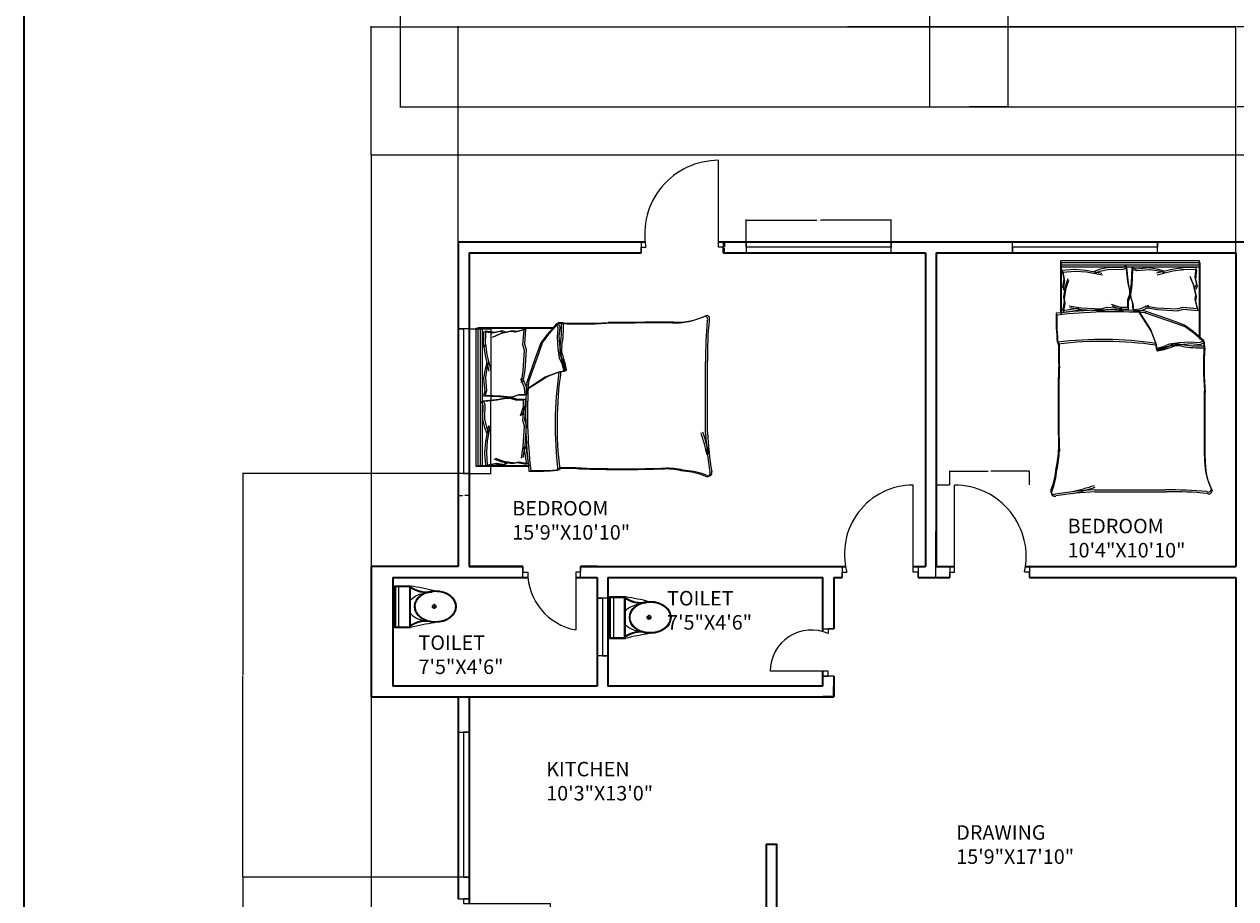
# Model space of a CAD drawing. Units: inches. Extents: x 1520 to 3401, y 1570 to 3432.
# Tile 5 of 15: x 1520 to 2022, y 2425 to 2787. Entities that reach past the tile are written whole.
import ezdxf

# ---------------------------------------------------------------- set-up
doc = ezdxf.new("R2010")
doc.units = ezdxf.units.IN
for name, color, linetype, lineweight in [('A-ANNO-DIMS', 2, 'Continuous', 18), ('A-ANNO-TTLB', 7, 'Continuous', 35), ('A-AREA-IDEN', 7, 'Continuous', 18), ('A-DOOR', 3, 'Continuous', 18), ('A-FLOR-EDGE', 7, 'Continuous', 25), ('A-FLOR-FIXT', 9, 'Continuous', 18), ('A-FURN', 8, 'Continuous', 13), ('A-GLAZ', 4, 'Continuous', 18), ('A-WALL', 7, 'Continuous', 35)]:
    doc.layers.add(name, color=color, linetype=linetype, lineweight=lineweight)
doc.styles.get("Standard").update_dxf_attribs({"font": 'arial.ttf'})
doc.dimstyles.get("Standard").update_dxf_attribs({"dimtxt": 0.18, "dimasz": 0.18, "dimexe": 0.18, "dimexo": 0.0625, "dimgap": 0.09, "dimtad": 0, "dimtih": 1, "dimtoh": 1, "dimdec": 4, "dimzin": 0, "dimdsep": 46, "dimtxsty": 'Standard', "dimcen": 0.09, "dimadec": 0, "dimazin": 0, "dimtfac": 1, "dimtdec": 4, "dimtofl": 0, "dimtmove": 0, "dimatfit": 3, "dimfxl": 1, "dimtolj": 1, "dimtzin": 0, "dimarcsym": 0})

# ---------------------------------------------------------------- blocks, each defined once
blk = doc.blocks.new('A$C31115884')
for p, q in [((283, 498), (223, 498)), ((258, 466), (258, 523)), ((0, 200), (0, 0)), ((520, 200), (0, 200)), ((10, 190), (10, 10)), ((510, 190), (10, 190)), ((510, 10), (510, 190)), ((520, 0), (520, 200)), ((510, 54), (0, 54)), ((10, 10), (510, 10)), ((0, 0), (520, 0))]:
    blk.add_line(p, q)
blk.add_circle((256, 496), 23.6)
for centre, radius, start, end in [((2778, -205), 2807, 165.4549, 171.7133), ((-295, 403), 365, 324.2091, 9.3499), ((-295, 403), 375, 324.2091, 9.3499), ((806, 403), 365, 170.6501, 215.7909), ((3237, 905), 2807, 188.2867, 194.5451), ((384, 406), 293, 190.2774, 224.1564), ((139, 406), 293, 315.8436, 2.6563), ((806, 403), 375, 179.2036, 215.7909)]:
    blk.add_arc(centre, radius, start, end)
blk.add_ellipse((256, 510), major_axis=(0, -261), ratio=0.772727)
blk.add_open_spline([(256, 259), (263, 259), (270, 260), (288, 262), (299, 265), (320, 273), (330, 278), (350, 291), (360, 299), (378, 316), (386, 326), (402, 347), (409, 358), (421, 383), (427, 395), (436, 422), (440, 436), (445, 465), (447, 480), (448, 509), (448, 524), (445, 553), (443, 568), (436, 596), (432, 610), (422, 636), (416, 649), (402, 672), (395, 683), (379, 703), (370, 712), (351, 728), (341, 735), (321, 746), (310, 751), (289, 757), (278, 759), (256, 761), (245, 761), (223, 757), (212, 754), (191, 746), (181, 741), (161, 728), (151, 720), (133, 703), (125, 693), (110, 672), (103, 660), (90, 636), (85, 623), (76, 596), (72, 582), (67, 553), (66, 538), (64, 509), (65, 494), (68, 465), (70, 450), (77, 422), (81, 408), (91, 382), (97, 370), (111, 346), (118, 335), (135, 316), (144, 307), (162, 291), (172, 284), (193, 273), (203, 269), (225, 262), (236, 260), (250, 259), (253, 259), (256, 259)], degree=3, knots=[0, 0, 0, 0, 0.110105, 0.110105, 0.285049, 0.285049, 0.459994, 0.459994, 0.634938, 0.634938, 0.809882, 0.809882, 0.984827, 0.984827, 1.159771, 1.159771, 1.334715, 1.334715, 1.50966, 1.50966, 1.684604, 1.684604, 1.859549, 1.859549, 2.034493, 2.034493, 2.209437, 2.209437, 2.384382, 2.384382, 2.559326, 2.559326, 2.73427, 2.73427, 2.909215, 2.909215, 3.084159, 3.084159, 3.259103, 3.259103, 3.434048, 3.434048, 3.608992, 3.608992, 3.783936, 3.783936, 3.958881, 3.958881, 4.133825, 4.133825, 4.30877, 4.30877, 4.483714, 4.483714, 4.658658, 4.658658, 4.833603, 4.833603, 5.008547, 5.008547, 5.183491, 5.183491, 5.358436, 5.358436, 5.53338, 5.53338, 5.708324, 5.708324, 5.883269, 5.883269, 6.058213, 6.058213, 6.233158, 6.233158, 6.283185, 6.283185, 6.283185, 6.283185])
blk = doc.blocks.new('DOOR-SWING-24-01')
for p, q in [((21.75, 19.61), (26.25, 19.61)), ((26.25, 19.61), (24, 19.61)), ((24, 19.61), (24, 17.61)), ((24, 2), (0, 2)), ((24, 0), (24, 2)), ((26.25, 0), (21.75, 0)), ((21.75, 0), (24, 0))]:
    blk.add_line(p, q)
blk.add_arc((17.08, 2), 17.08, 66.0978, 180)
blk = doc.blocks.new('DOOR-SWING-24-02')
for p, q in [((0, 21.75), (0, 26.25)), ((0, 26.25), (0, 24)), ((23.89, 21.75), (23.89, 26.25)), ((23.89, 26.25), (23.89, 24)), ((0, 24), (2, 24)), ((23.89, 24), (21.89, 24)), ((21.89, 24), (21.89, 0))]:
    blk.add_line(p, q)
blk.add_arc((26.42, 24), 24.42, 180, 259.3013)
blk = doc.blocks.new('DOOR-SWING-36-03')
for p, q in [((29.45, 2.25), (29.45, 38.25)), ((0, 4.5), (0, 0)), ((0, 0), (0, 2.25)), ((0, 2.25), (2, 2.25)), ((31.45, 2.25), (29.45, 2.25)), ((31.45, 4.5), (31.45, 0)), ((31.45, 0), (31.45, 2.25))]:
    blk.add_line(p, q)
blk.add_arc((29.45, 9.79), 28.46, 90, 195.3561)
blk = doc.blocks.new('DOOR-SWING-36-04')
for p, q in [((2, 2.25), (2, 38.25)), ((0, 4.5), (0, 0)), ((0, 0), (0, 2.25)), ((0, 2.25), (2, 2.25)), ((32.99, 2.25), (30.99, 2.25)), ((32.99, 4.5), (32.99, 0)), ((32.99, 0), (32.99, 2.25))]:
    blk.add_line(p, q)
blk.add_arc((2, 8.58), 29.67, 347.6919, 90)
blk = doc.blocks.new('DOOR-SWING-36-22')
for p, q in [((32.08, 2.25), (32.08, 38.25)), ((0, 4.5), (0, 0)), ((0, 0), (0, 2.25)), ((0, 2.25), (2, 2.25)), ((34.08, 2.25), (32.08, 2.25)), ((34.08, 4.5), (34.08, 0)), ((34.08, 0), (34.08, 2.25))]:
    blk.add_line(p, q)
blk.add_arc((32.08, 7.69), 30.56, 90, 190.2449)
blk = doc.blocks.new('DOOR-SWING-36-24')
for p, q in [((0, 30.42), (4.5, 30.42)), ((4.5, 30.42), (2.25, 30.42)), ((2.25, 30.42), (2.25, 28.42)), ((2.25, 28.42), (38.25, 28.42)), ((4.5, 0), (0, 0)), ((0, 0), (2.25, 0)), ((2.25, 0), (2.25, 2))]:
    blk.add_line(p, q)
blk.add_arc((10.55, 28.42), 27.7, 252.5577, 0)
blk = doc.blocks.new('WIN-PLAN-24-01')
for p, q in [((0, 4.5), (0, 0)), ((0, 0), (0, 2.25)), ((0, 2.25), (24, 2.25)), ((24, 2.25), (24, 4.5)), ((24, 4.5), (24, 0))]:
    blk.add_line(p, q)
blk = doc.blocks.new('WIN-PLAN-60-02')
for p, q in [((4.5, 60), (0, 60)), ((0, 60), (2.25, 60)), ((2.25, 60), (2.25, 0)), ((4.5, 0), (0, 0)), ((2.25, 0), (4.5, 0))]:
    blk.add_line(p, q)
blk = doc.blocks.new('WIN-PLAN-60-03')
for p, q in [((0, 2.25), (0, 4.5)), ((0, 4.5), (0, 0)), ((60, 2.25), (0, 2.25)), ((60, 0), (60, 4.5)), ((60, 4.5), (60, 2.25))]:
    blk.add_line(p, q)
blk = doc.blocks.new('BED-DOUBLE')
for p, q in [((4.17, 75.93), (4.17, 97.64)), ((4.17, 97.64), (61.46, 97.64)), ((4.17, 95.8), (61.46, 95.8)), ((4.44, 75.16), (4.44, 96.87)), ((4.44, 96.87), (61.73, 96.87)), ((29.42, 94.7), (31.15, 95.4)), ((31.15, 95.4), (31.84, 88.98)), ((61.46, 97.64), (61.46, 65.74)), ((61.73, 96.87), (61.73, 64.97)), ((4.44, 95.03), (61.73, 95.03)), ((4.67, 93.64), (9.81, 94.03)), ((4.67, 93.66), (5.36, 89.85)), ((4.94, 92.9), (5.64, 89.08)), ((4.95, 92.87), (10.08, 93.27)), ((9.81, 94.03), (9.93, 94.01)), ((9.93, 94.01), (14.52, 93.66)), ((10.08, 93.27), (10.21, 93.24)), ((10.21, 93.24), (14.79, 92.9)), ((14.52, 93.66), (21.1, 92.45)), ((14.79, 92.9), (21.38, 91.68)), ((17.81, 93.14), (20.24, 94.01)), ((18.08, 92.38), (20.51, 93.24)), ((20.24, 94.01), (23.7, 94.88)), ((20.51, 93.24), (23.98, 94.11)), ((23.7, 94.88), (24.09, 94.88)), ((23.98, 94.11), (24.36, 94.11)), ((24.09, 94.88), (29.42, 94.7)), ((24.36, 94.11), (29.69, 93.94)), ((29.69, 93.94), (31.42, 94.63)), ((31.42, 94.63), (32.12, 88.22)), ((33.54, 94.65), (33.25, 88.21)), ((33.81, 93.88), (33.52, 87.44)), ((35.31, 94.07), (33.54, 94.65)), ((35.59, 93.3), (33.81, 93.88)), ((40.62, 94.57), (35.31, 94.07)), ((40.9, 93.81), (35.59, 93.3)), ((41.01, 94.6), (40.62, 94.57)), ((41.28, 93.83), (40.9, 93.81)), ((44.52, 93.95), (41.01, 94.6)), ((44.79, 93.18), (41.28, 93.83)), ((50.25, 93.96), (43.75, 92.34)), ((50.52, 93.19), (44.03, 91.57)), ((47, 93.23), (44.52, 93.95)), ((47.27, 92.47), (44.79, 93.18)), ((54.8, 94.59), (50.25, 93.96)), ((55.08, 93.82), (50.52, 93.19)), ((60.08, 94.57), (53.6, 94.69)), ((53.6, 94.69), (54.8, 94.59)), ((60.35, 93.81), (53.87, 93.92)), ((53.87, 93.92), (55.08, 93.82)), ((59.12, 87.74), (57.7, 90.95)), ((60.08, 94.57), (59.62, 90.72)), ((59.62, 90.72), (60.34, 87.64)), ((60.35, 93.81), (59.9, 89.96)), ((5.36, 89.85), (4.84, 86.73)), ((4.84, 86.73), (5.54, 85.52)), ((5.64, 89.08), (5.12, 85.96)), ((5.12, 85.96), (5.81, 84.75)), ((5.36, 82.57), (6.06, 86.9)), ((5.64, 81.8), (6.33, 86.14)), ((6.06, 86.9), (7.27, 90.2)), ((6.33, 86.14), (7.54, 89.43)), ((31.84, 88.98), (32.54, 85.17)), ((32.12, 88.22), (32.81, 84.4)), ((33.25, 88.21), (32.79, 84.36)), ((33.52, 87.44), (33.07, 83.59)), ((59.39, 86.97), (57.97, 90.18)), ((60.08, 83.46), (59.12, 87.74)), ((60.35, 82.69), (59.39, 86.97)), ((60.34, 87.64), (59.72, 86.39)), ((59.9, 89.96), (60.61, 86.88)), ((60.61, 86.88), (59.99, 85.62)), ((5.02, 76.85), (5.71, 80.66)), ((5.71, 80.66), (5.36, 82.57)), ((5.98, 79.9), (5.64, 81.8)), ((32.54, 83.61), (31.84, 81.36)), ((31.84, 81.36), (31.84, 78.14)), ((32.81, 82.84), (32.12, 80.59)), ((32.12, 80.59), (32.12, 77.37)), ((32.54, 85.17), (32.54, 83.61)), ((32.79, 84.36), (32.89, 82.8)), ((32.81, 84.4), (32.81, 82.84)), ((32.89, 82.8), (33.72, 80.59)), ((33.07, 83.59), (33.17, 82.03)), ((33.17, 82.03), (34, 79.83)), ((33.72, 80.59), (33.93, 77.39)), ((59.85, 81.53), (60.08, 83.46)), ((60.78, 77.77), (59.85, 81.53)), ((60.12, 80.77), (60.35, 82.69)), ((61.05, 77), (60.12, 80.77)), ((11.13, 77.72), (5.02, 76.85)), ((5.29, 76.08), (5.98, 79.9)), ((11.4, 76.95), (5.29, 76.08)), ((7.65, 78.9), (12.48, 78.1)), ((7.92, 78.14), (12.76, 77.34)), ((12.48, 78.1), (11.13, 77.72)), ((12.76, 77.34), (11.4, 76.95)), ((12.48, 78.1), (20.89, 77.59)), ((12.76, 77.34), (21.16, 76.82)), ((20.89, 77.59), (23.24, 78.25)), ((21.16, 76.82), (23.51, 77.49)), ((23.24, 78.25), (29.39, 77.77)), ((23.51, 77.49), (29.67, 77)), ((28.9, 78.14), (25.13, 79.45)), ((29.17, 77.37), (25.4, 78.68)), ((31.84, 78.14), (28.9, 78.14)), ((32.12, 77.37), (29.17, 77.37)), ((33.93, 77.39), (36.87, 77.57)), ((34, 79.83), (34.2, 76.62)), ((34.2, 76.62), (37.14, 76.8)), ((36.28, 76.8), (41.3, 69.01)), ((36.55, 76.03), (41.57, 68.25)), ((36.87, 77.57), (40.55, 79.11)), ((37.14, 76.8), (40.82, 78.34)), ((48.73, 73.28), (38.73, 76.8)), ((49, 72.52), (39, 76.03)), ((39.04, 78.9), (43.87, 78.1)), ((39.31, 78.14), (44.15, 77.34)), ((43.87, 78.1), (52.28, 77.59)), ((44.15, 77.34), (52.55, 76.82)), ((52.28, 77.59), (54.63, 78.25)), ((52.55, 76.82), (54.9, 77.49)), ((54.63, 78.25), (60.78, 77.77)), ((54.9, 77.49), (61.05, 77)), ((55.41, 70.87), (48.73, 73.28)), ((55.69, 70.1), (49, 72.52)), ((58.94, 68.27), (55.41, 70.87)), ((41.3, 69.01), (43.34, 63.63)), ((41.57, 68.25), (43.62, 62.87)), ((59.21, 67.51), (55.69, 70.1)), ((63.38, 64.38), (58.94, 68.27)), ((63.66, 63.61), (59.21, 67.51)), ((43.34, 63.63), (43.71, 61.22)), ((43.62, 62.87), (43.99, 60.45)), ((43.71, 61.22), (46.68, 61.96)), ((43.99, 60.45), (46.96, 61.2)), ((46.68, 61.96), (49.1, 63.08)), ((46.96, 61.2), (49.37, 62.31)), ((49.1, 63.08), (53.18, 63.63)), ((49.37, 62.31), (53.46, 62.87)), ((53.18, 63.63), (57.82, 64)), ((53.46, 62.87), (58.1, 63.24)), ((57.82, 64), (61.54, 63.63)), ((58.1, 63.24), (61.81, 62.87)), ((61.54, 63.63), (63.38, 64.38)), ((61.81, 62.87), (63.66, 63.61)), ((63.48, 62.28), (63.38, 64.38, 4.64)), ((63.75, 61.52), (63.66, 63.61, 4.64)), ((18.06, 2.64), (47.57, 2.64)), ((18.33, 1.87), (47.84, 1.87))]:
    blk.add_line(p, q)
for centre, radius, start, end in [((102.1, 73.55), 99.87, 178.7218, 185.604), ((25.61, -120.62), 197.77, 86.0865, 96.7821), ((25.88, -121.38), 197.77, 86.0865, 96.7821), ((102.37, 72.78), 99.87, 178.7218, 185.604), ((21.29, -89.76), 154.68, 81.7845, 96.9006), ((21.56, -90.53), 154.68, 81.7845, 96.9006), ((-200.58, 60.27), 203.94, 358.4762, 1.0082), ((-200.3, 59.5), 203.94, 358.4762, 1.0082), ((43.92, 61.15), 0.221, 160.2464, 271.1377), ((37.35, 95.86), 35.55, 280.6617, 289.8806), ((44.2, 60.38), 0.221, 160.2464, 271.1377), ((37.62, 95.1), 35.55, 280.6617, 289.8806), ((52.44, 55.6), 7.46, 78.6608, 113.7384), ((52.72, 54.83), 7.46, 78.6608, 113.7384), ((61.53, 105.62), 43.38, 259.8763, 272.5657), ((61.81, 104.85), 43.38, 259.8763, 272.5657), ((218.51, 54.1), 155.25, 176.9791, 183.8365), ((218.79, 53.34), 155.25, 176.9791, 183.8365), ((581.23, 36.96), 578.22, 178.22771, 181.71854), ((581.51, 36.19), 578.22, 178.22771, 181.71854), ((-5405.34, 16.33), 5469.02, 0.00217, 0.28689), ((-5405.07, 15.56), 5469.02, 0.00217, 0.28689), ((-32.25, 20.29), 35.53, 346.0648, 358.9113), ((-31.97, 19.53), 35.53, 346.0648, 358.9113), ((91.3, 15.32), 27.65, 177.4714, 206.4681), ((91.58, 14.55), 27.65, 177.4714, 206.4681), ((-25.97, 13.39), 28.25, 337.9751, 356.652), ((-25.69, 12.62), 28.25, 337.9751, 356.652), ((1.3, 2.07), 1.31, 146.1736, 293.4781), ((1.58, 1.3), 1.31, 146.1736, 293.4781), ((25.69, -143.14), 145.97, 92.9958, 99.4091), ((25.96, -143.9), 145.97, 92.9958, 99.4091), ((-20.65, 126.07), 127.63, 283.3832, 287.7053), ((-20.37, 125.3), 127.63, 283.3832, 287.7053), ((49.34, -156.85), 159.5, 84.4998, 90.6351), ((49.61, -157.62), 159.5, 84.4998, 90.6351), ((65.23, 3.08), 1.32, 242.6588, 356.02), ((65.5, 2.32), 1.32, 242.6588, 356.02)]:
    blk.add_arc(centre, radius, start, end)
blk = doc.blocks.new('*D61')
at = {"layer": 'A-ANNO-DIMS', "color": 0, "lineweight": -2, "transparency": 16777216}
for p, q in [((1704.18, 2661.18), (1713.29, 2661.18)), ((1713.11, 2661), (1713.11, 2631.37)), ((1713.11, 2601.36), (1713.11, 2631)), ((1704.18, 2601.18), (1713.29, 2601.18))]:
    blk.add_line(p, q, dxfattribs=at)
at = {"layer": 'A-ANNO-DIMS', "color": 0, "transparency": 16777216}
for points in [[(1713.08, 2661), (1713.14, 2661), (1713.11, 2661.18)], [(1713.08, 2601.36), (1713.14, 2601.36), (1713.11, 2601.18)]]:
    blk.add_solid(points, dxfattribs=at)
at = {"layer": 'Defpoints', "color": 0, "transparency": 16777216}
for p in [(1704.11, 2661.18), (1713.11, 2661.18), (1704.11, 2601.18)]:
    blk.add_point(p, dxfattribs=at)
at = {"layer": 'A-ANNO-DIMS', "color": 0, "transparency": 16777216, "insert": (1713.11, 2631.18), "char_height": 0.18, "attachment_point": 5}
blk.add_mtext('\\A1;W2 60 TYP.', dxfattribs=at)
blk = doc.blocks.new('*D62')
at = {"layer": 'A-ANNO-DIMS', "color": 0, "lineweight": -2, "transparency": 16777216}
for p, q in [((1699.61, 2601.12), (1699.61, 2592)), ((1704.11, 2601.12), (1704.11, 2592)), ((1699.79, 2592.18), (1701.4, 2592.18)), ((1703.93, 2592.18), (1702.32, 2592.18))]:
    blk.add_line(p, q, dxfattribs=at)
at = {"layer": 'A-ANNO-DIMS', "color": 0, "transparency": 16777216}
for points in [[(1699.79, 2592.21), (1699.79, 2592.15), (1699.61, 2592.18)], [(1703.93, 2592.21), (1703.93, 2592.15), (1704.11, 2592.18)]]:
    blk.add_solid(points, dxfattribs=at)
at = {"layer": 'Defpoints', "color": 0, "transparency": 16777216}
for p in [(1699.61, 2601.18), (1704.11, 2601.18), (1704.11, 2592.18)]:
    blk.add_point(p, dxfattribs=at)
at = {"layer": 'A-ANNO-DIMS', "color": 0, "transparency": 16777216, "insert": (1701.86, 2592.18), "char_height": 0.18, "attachment_point": 5}
blk.add_mtext('\\A1;5 TYP.', dxfattribs=at)
blk = doc.blocks.new('*D65')
at = {"layer": 'A-ANNO-DIMS', "color": 0, "lineweight": -2, "transparency": 16777216}
for p, q in [((1818.93, 2697.24), (1818.93, 2706.36)), ((1819.11, 2706.18), (1848.18, 2706.18)), ((1878.75, 2706.18), (1849.69, 2706.18)), ((1878.93, 2697.24), (1878.93, 2706.36))]:
    blk.add_line(p, q, dxfattribs=at)
at = {"layer": 'A-ANNO-DIMS', "color": 0, "transparency": 16777216}
for points in [[(1819.11, 2706.21), (1819.11, 2706.15), (1818.93, 2706.18)], [(1878.75, 2706.21), (1878.75, 2706.15), (1878.93, 2706.18)]]:
    blk.add_solid(points, dxfattribs=at)
at = {"layer": 'Defpoints', "color": 0, "transparency": 16777216}
for p in [(1878.93, 2706.18), (1818.93, 2697.18), (1878.93, 2697.18)]:
    blk.add_point(p, dxfattribs=at)
at = {"layer": 'A-ANNO-DIMS', "color": 0, "transparency": 16777216, "insert": (1848.93, 2706.18), "char_height": 0.18, "attachment_point": 5}
blk.add_mtext('\\A1;W3 60 TYP.', dxfattribs=at)
blk = doc.blocks.new('*D66')
at = {"layer": 'A-ANNO-DIMS', "color": 0, "lineweight": -2, "transparency": 16777216}
for p, q in [((1818.87, 2697.18), (1809.75, 2697.18)), ((1809.93, 2697), (1809.93, 2695.11)), ((1809.93, 2692.86), (1809.93, 2694.75)), ((1818.87, 2692.68), (1809.75, 2692.68))]:
    blk.add_line(p, q, dxfattribs=at)
at = {"layer": 'A-ANNO-DIMS', "color": 0, "transparency": 16777216}
for points in [[(1809.9, 2697), (1809.96, 2697), (1809.93, 2697.18)], [(1809.9, 2692.86), (1809.96, 2692.86), (1809.93, 2692.68)]]:
    blk.add_solid(points, dxfattribs=at)
at = {"layer": 'Defpoints', "color": 0, "transparency": 16777216}
for p in [(1809.93, 2697.18), (1818.93, 2697.18), (1818.93, 2692.68)]:
    blk.add_point(p, dxfattribs=at)
at = {"layer": 'A-ANNO-DIMS', "color": 0, "transparency": 16777216, "insert": (1809.93, 2694.93), "char_height": 0.18, "attachment_point": 5}
blk.add_mtext('\\A1;5 TYP.', dxfattribs=at)
blk = doc.blocks.new('*D87')
at = {"layer": 'A-ANNO-DIMS', "color": 0, "lineweight": -2, "transparency": 16777216}
for p, q in [((1903.1, 2596.43), (1897.25, 2596.43)), ((1897.43, 2596.25), (1897.43, 2577.49)), ((1897.43, 2558.36), (1897.43, 2577.12)), ((1903.1, 2558.18), (1897.25, 2558.18))]:
    blk.add_line(p, q, dxfattribs=at)
at = {"layer": 'A-ANNO-DIMS', "color": 0, "transparency": 16777216}
for points in [[(1897.4, 2596.25), (1897.46, 2596.25), (1897.43, 2596.43)], [(1897.4, 2558.36), (1897.46, 2558.36), (1897.43, 2558.18)]]:
    blk.add_solid(points, dxfattribs=at)
at = {"layer": 'Defpoints', "color": 0, "transparency": 16777216}
for p in [(1897.43, 2596.43), (1903.16, 2596.43), (1903.16, 2558.18)]:
    blk.add_point(p, dxfattribs=at)
at = {"layer": 'A-ANNO-DIMS', "color": 0, "transparency": 16777216, "insert": (1897.43, 2577.3), "char_height": 0.18, "attachment_point": 5}
blk.add_mtext('\\A1;D04 38 TYP.', dxfattribs=at)
blk = doc.blocks.new('*D88')
at = {"layer": 'A-ANNO-DIMS', "color": 0, "lineweight": -2, "transparency": 16777216}
for p, q in [((1903.16, 2596.49), (1903.16, 2602.35)), ((1903.34, 2602.17), (1919.13, 2602.17)), ((1935.98, 2602.17), (1920.19, 2602.17)), ((1936.16, 2596.49), (1936.16, 2602.35))]:
    blk.add_line(p, q, dxfattribs=at)
at = {"layer": 'A-ANNO-DIMS', "color": 0, "transparency": 16777216}
for points in [[(1903.34, 2602.2), (1903.34, 2602.14), (1903.16, 2602.17)], [(1935.98, 2602.2), (1935.98, 2602.14), (1936.16, 2602.17)]]:
    blk.add_solid(points, dxfattribs=at)
at = {"layer": 'Defpoints', "color": 0, "transparency": 16777216}
for p in [(1936.16, 2602.17), (1903.16, 2596.43), (1936.16, 2596.43)]:
    blk.add_point(p, dxfattribs=at)
at = {"layer": 'A-ANNO-DIMS', "color": 0, "transparency": 16777216, "insert": (1919.66, 2602.17), "char_height": 0.18, "attachment_point": 5}
blk.add_mtext('\\A1;33 TYP.', dxfattribs=at)
blk = doc.blocks.new('*D181')
at = {"layer": 'A-ANNO-DIMS', "color": 0, "lineweight": -2, "transparency": 16777216}
for p, q in [((1663.61, 2733.24), (1663.61, 2786.46)), ((1663.79, 2786.28), (2021.47, 2786.28)), ((2379.93, 2786.28), (2022.26, 2786.28)), ((2380.11, 2733.24), (2380.11, 2786.46))]:
    blk.add_line(p, q, dxfattribs=at)
at = {"layer": 'A-ANNO-DIMS', "color": 0, "transparency": 16777216}
for points in [[(1663.79, 2786.31), (1663.79, 2786.25), (1663.61, 2786.28)], [(2379.93, 2786.31), (2379.93, 2786.25), (2380.11, 2786.28)]]:
    blk.add_solid(points, dxfattribs=at)
at = {"layer": 'Defpoints', "color": 0, "transparency": 16777216}
for p in [(2380.11, 2786.28), (1663.61, 2733.18), (2380.11, 2733.18)]:
    blk.add_point(p, dxfattribs=at)
at = {"layer": 'A-ANNO-DIMS', "color": 0, "transparency": 16777216, "insert": (2021.86, 2786.28), "char_height": 0.18, "attachment_point": 5}
blk.add_mtext('\\A1;716.5', dxfattribs=at)
blk = doc.blocks.new('*D183')
at = {"layer": 'A-ANNO-DIMS', "color": 0, "lineweight": -2, "transparency": 16777216}
for p, q in [((1699.61, 2697.24), (1699.61, 2786.46)), ((1699.79, 2786.28), (1860.32, 2786.28)), ((2021.43, 2786.28), (1860.9, 2786.28)), ((2021.61, 2692.74), (2021.61, 2786.46))]:
    blk.add_line(p, q, dxfattribs=at)
at = {"layer": 'A-ANNO-DIMS', "color": 0, "transparency": 16777216}
for points in [[(1699.79, 2786.31), (1699.79, 2786.25), (1699.61, 2786.28)], [(2021.43, 2786.31), (2021.43, 2786.25), (2021.61, 2786.28)]]:
    blk.add_solid(points, dxfattribs=at)
at = {"layer": 'Defpoints', "color": 0, "transparency": 16777216}
for p in [(2021.61, 2786.28), (1699.61, 2697.18), (2021.61, 2692.68)]:
    blk.add_point(p, dxfattribs=at)
at = {"layer": 'A-ANNO-DIMS', "color": 0, "transparency": 16777216, "insert": (1860.61, 2786.28), "char_height": 0.18, "attachment_point": 5}
blk.add_mtext('\\A1;322', dxfattribs=at)
blk = doc.blocks.new('*D190')
at = {"layer": 'A-ANNO-DIMS', "color": 0, "lineweight": -2, "transparency": 16777216}
for p, q in [((1699.55, 2434.03), (1610.33, 2434.03)), ((1610.51, 2433.85), (1610.51, 2414.53)), ((1610.51, 2394.85), (1610.51, 2414.17)), ((1699.55, 2394.67), (1610.33, 2394.67))]:
    blk.add_line(p, q, dxfattribs=at)
at = {"layer": 'A-ANNO-DIMS', "color": 0, "transparency": 16777216}
for points in [[(1610.48, 2433.85), (1610.54, 2433.85), (1610.51, 2434.03)], [(1610.48, 2394.85), (1610.54, 2394.85), (1610.51, 2394.67)]]:
    blk.add_solid(points, dxfattribs=at)
at = {"layer": 'Defpoints', "color": 0, "transparency": 16777216}
for p in [(1610.51, 2434.03), (1699.61, 2434.03), (1699.61, 2394.67)]:
    blk.add_point(p, dxfattribs=at)
at = {"layer": 'A-ANNO-DIMS', "color": 0, "transparency": 16777216, "insert": (1610.51, 2414.35), "char_height": 0.18, "attachment_point": 5}
blk.add_mtext('\\A1;39.36', dxfattribs=at)
blk = doc.blocks.new('*D191')
at = {"layer": 'A-ANNO-DIMS', "color": 0, "lineweight": -2, "transparency": 16777216}
for p, q in [((1699.55, 2601.18), (1610.33, 2601.18)), ((1610.51, 2601), (1610.51, 2517.79)), ((1610.51, 2434.21), (1610.51, 2517.43)), ((1699.55, 2434.03), (1610.33, 2434.03))]:
    blk.add_line(p, q, dxfattribs=at)
at = {"layer": 'A-ANNO-DIMS', "color": 0, "transparency": 16777216}
for points in [[(1610.48, 2601), (1610.54, 2601), (1610.51, 2601.18)], [(1610.48, 2434.21), (1610.54, 2434.21), (1610.51, 2434.03)]]:
    blk.add_solid(points, dxfattribs=at)
at = {"layer": 'Defpoints', "color": 0, "transparency": 16777216}
for p in [(1610.51, 2601.18), (1699.61, 2601.18), (1699.61, 2434.03)]:
    blk.add_point(p, dxfattribs=at)
at = {"layer": 'A-ANNO-DIMS', "color": 0, "transparency": 16777216, "insert": (1610.51, 2517.61), "char_height": 0.18, "attachment_point": 5}
blk.add_mtext('\\A1;167.15', dxfattribs=at)
blk = doc.blocks.new('*D209')
at = {"layer": 'A-ANNO-DIMS', "color": 0, "lineweight": -2, "transparency": 16777216}
for p, q in [((1675.61, 3007.57), (1675.61, 2752.86)), ((2368.11, 3007.57), (2368.11, 2752.86)), ((1675.79, 2753.04), (2021.47, 2753.04)), ((2367.93, 2753.04), (2022.26, 2753.04))]:
    blk.add_line(p, q, dxfattribs=at)
at = {"layer": 'A-ANNO-DIMS', "color": 0, "transparency": 16777216}
for points in [[(1675.79, 2753.07), (1675.79, 2753.01), (1675.61, 2753.04)], [(2367.93, 2753.07), (2367.93, 2753.01), (2368.11, 2753.04)]]:
    blk.add_solid(points, dxfattribs=at)
at = {"layer": 'Defpoints', "color": 0, "transparency": 16777216}
for p in [(1675.61, 3007.63), (2368.11, 3007.63), (2368.11, 2753.04)]:
    blk.add_point(p, dxfattribs=at)
at = {"layer": 'A-ANNO-DIMS', "color": 0, "transparency": 16777216, "insert": (2021.86, 2753.04), "char_height": 0.18, "attachment_point": 5}
blk.add_mtext('\\A1;692.5', dxfattribs=at)
blk = doc.blocks.new('*D214')
at = {"layer": 'A-ANNO-DIMS', "color": 0, "lineweight": -2, "transparency": 16777216}
for p, q in [((1894.73, 2881.57), (1894.73, 2752.86)), ((1927.22, 2881.57), (1927.22, 2752.86)), ((1894.91, 2753.04), (1910.58, 2753.04)), ((1927.04, 2753.04), (1911.37, 2753.04))]:
    blk.add_line(p, q, dxfattribs=at)
at = {"layer": 'A-ANNO-DIMS', "color": 0, "transparency": 16777216}
for points in [[(1894.91, 2753.07), (1894.91, 2753.01), (1894.73, 2753.04)], [(1927.04, 2753.07), (1927.04, 2753.01), (1927.22, 2753.04)]]:
    blk.add_solid(points, dxfattribs=at)
at = {"layer": 'Defpoints', "color": 0, "transparency": 16777216}
for p in [(1894.73, 2881.63), (1927.22, 2881.63), (1927.22, 2753.04)]:
    blk.add_point(p, dxfattribs=at)
at = {"layer": 'A-ANNO-DIMS', "color": 0, "transparency": 16777216, "insert": (1910.97, 2753.04), "char_height": 0.18, "attachment_point": 5}
blk.add_mtext('\\A1;32.49', dxfattribs=at)

msp = doc.modelspace()

# ---------------------------------------------------------------- linework, layer by layer
at = {"layer": 'A-ANNO-TTLB'}
msp.add_lwpolyline([(1519.9253, 3431.7421), (3400.8761, 3431.7421), (3400.8761, 1570.3458), (1519.9253, 1570.3458)], close=True, dxfattribs=at)
at = {"layer": 'A-FLOR-EDGE'}
for q in [(1663.6128, 1791.6786), (2380.1128, 2733.1786)]:
    msp.add_line((1663.6128, 2733.1786), q, dxfattribs=at)
at = {"layer": 'A-WALL'}
for p, q in [((1699.6128, 2697.1786), (1699.6128, 2562.6786)), ((1699.6128, 2697.1786), (1699.6128, 2562.6786)), ((1699.6128, 2697.1786), (1777.0094, 2697.1786)), ((1807.4069, 2697.1786), (2083.3571, 2697.1786)), ((1704.1128, 2692.6786), (1775.3302, 2692.6786)), ((1704.1128, 2692.6786), (1704.1128, 2562.6786)), ((1809.4069, 2692.6786), (1893.1128, 2692.6786)), ((1893.1128, 2692.6786), (1893.1128, 2562.6786)), ((1897.6128, 2692.6786), (1897.6128, 2562.6786)), ((1897.6128, 2692.6786), (2021.6128, 2692.6786)), ((2021.6128, 2692.6786), (2021.6128, 2562.6786)), ((1663.6128, 2562.6786), (1663.6128, 2508.6786)), ((1699.6128, 2562.6786), (1663.6128, 2562.6786)), ((1704.1128, 2562.6786), (1726.4191, 2562.6786)), ((1726.4191, 2562.6786), (1704.1128, 2562.6786)), ((1757.1128, 2562.6786), (1750.3094, 2562.6786)), ((1750.3094, 2562.6786), (1860.0654, 2562.6786)), ((1888.0326, 2562.6786), (1893.1128, 2562.6786)), ((1897.6128, 2562.6786), (1905.1643, 2562.6786)), ((1934.5575, 2562.6786), (2021.6128, 2562.6786)), ((1672.6128, 2558.1786), (1728.523, 2558.1786)), ((1672.6128, 2558.1786), (1672.6128, 2513.1786)), ((1748.3094, 2558.1786), (1757.1128, 2558.1786)), ((1757.1128, 2558.1786), (1757.1128, 2513.1786)), ((1761.6128, 2558.1786), (1761.6128, 2513.1786)), ((1761.6128, 2558.1786), (1850.6128, 2558.1786)), ((1850.6128, 2535.7697), (1850.6128, 2558.1786)), ((1855.1128, 2558.1786), (1855.1128, 2536.9559)), ((1855.1128, 2558.1786), (1858.5861, 2558.1786)), ((1890.0326, 2558.1786), (1903.1643, 2558.1786)), ((1936.1567, 2558.1786), (2021.6128, 2558.1786)), ((2021.6128, 2558.1786), (2021.6128, 2343.1786)), ((1850.6128, 2513.1786), (1850.6128, 2519.341)), ((1855.1128, 2517.341), (1855.1128, 2508.6786)), ((1663.6128, 2508.6786), (1761.6128, 2508.6786)), ((1757.1128, 2513.1786), (1672.6128, 2513.1786)), ((1699.6128, 2508.6786), (1699.6128, 2425.0977)), ((1699.6128, 2508.6786), (1699.6128, 2425.0977)), ((1704.1128, 2508.6786), (1704.1128, 2423.0977)), ((1704.1128, 2508.6786), (1827.1128, 2508.6786)), ((1850.6128, 2513.1786), (1761.6128, 2513.1786)), ((1761.6128, 2508.6786), (1827.1128, 2508.6786)), ((1827.1128, 2508.6786), (1831.6128, 2508.6786)), ((1831.6128, 2508.6786), (1850.6128, 2508.6786)), ((1855.1128, 2508.6786), (1850.6128, 2508.6786)), ((1850.6128, 2508.6786), (1855.1128, 2508.6786)), ((1855.1128, 2508.6786), (1855.1128, 2513.1786)), ((1827.1128, 2447.697), (1827.1128, 2343.1786)), ((1827.1128, 2447.697), (1831.6128, 2447.697)), ((1831.6128, 2343.1786), (1831.6128, 2447.697))]:
    msp.add_line(p, q, dxfattribs=at)

# ---------------------------------------------------------------- block references
at = {"layer": 'A-DOOR'}
for name, p in [('DOOR-SWING-36-22', (1775.33, 2692.679)), ('DOOR-SWING-36-03', (1858.586, 2558.179)), ('DOOR-SWING-36-04', (1903.164, 2558.179)), ('DOOR-SWING-24-02', (1726.419, 2536.429)), ('DOOR-SWING-24-01', (1828.863, 2517.341)), ('DOOR-SWING-36-24', (1699.613, 2394.673))]:
    msp.add_blockref(name, p, dxfattribs=at)
at = {"layer": 'A-FLOR-FIXT', "xscale": 0.0330640103915726, "yscale": 0.0330640103915726, "zscale": 0.0330640103915726, "rotation": 270}
for p in [(1673.3037, 2554.5886), (1762.2647, 2550.1138)]:
    msp.add_blockref('A$C31115884', p, dxfattribs=at)
at = {"layer": 'A-FURN'}
msp.add_blockref('BED-DOUBLE', (1945.003, 2591.804), dxfattribs=at)
at = {"layer": 'A-FURN', "rotation": 90.00000000000003}
msp.add_blockref('BED-DOUBLE', (1804.6991, 2599.9003), dxfattribs=at)
at = {"layer": 'A-GLAZ'}
for name, p in [('WIN-PLAN-60-03', (1818.9306, 2692.679)), ('WIN-PLAN-60-02', (1699.613, 2601.185))]:
    msp.add_blockref(name, p, dxfattribs=at)
at = {"layer": 'A-GLAZ', "rotation": 270}
for name, p in [('WIN-PLAN-60-02', (1929.2102, 2697.1785)), ('WIN-PLAN-24-01', (1757.1132, 2549.6622))]:
    msp.add_blockref(name, p, dxfattribs=at)
at = {"layer": 'A-GLAZ', "extrusion": (0, 0, -1), "zscale": -1, "rotation": 90}
msp.add_blockref('WIN-PLAN-60-03', (-1699.6132, 2434.0305), dxfattribs=at)

# ---------------------------------------------------------------- texts
at = {"layer": 'A-AREA-IDEN', "char_height": 6, "attachment_point": 1}
for s, width, insert in [('BEDROOM\\P15\'9"X10\'10"', 117.959755, (1722.0111, 2589.8373)), ('BEDROOM\\P10\'4"X10\'10"', 101.124729, (1951.9731, 2582.4753)), ('TOILET\\P7\'5"X4\'6"', 88.670473, (1786.1367, 2552.5788)), ('TOILET\\P7\'5"X4\'6"', 78.425769, (1683.1871, 2534.1783)), ('KITCHEN\\P10\'3"X13\'0"', 158.525452, (1736.0739, 2481.8121)), ('DRAWING\\P15\'9"X17\'10"', 99.721211, (1905.8661, 2455.5581))]:
    msp.add_mtext_dynamic_manual_height_columns(s, width=width, gutter_width=12.5, heights=[0], dxfattribs=dict(at, insert=insert))

# ---------------------------------------------------------------- dimensions: what is measured, and where the dimension line sits
at = {"layer": 'A-ANNO-DIMS'}
for base, p1, p2, override, picture, middle in [((2368.1128, 2753.0384), (1675.6128, 3007.633), (2368.1128, 3007.633), {"dimdec": 1, "dimlfac": 1, "dimrnd": 0, "dimzin": 0, "dimdsep": 46, "dimlunit": 2}, '*D209', (2021.8628, 2753.0384)), ((1927.2204, 2753.0384), (1894.7277, 2881.633), (1927.2204, 2881.633), {"dimdec": 2, "dimlfac": 1, "dimrnd": 0, "dimzin": 0, "dimdsep": 46, "dimlunit": 2}, '*D214', (1910.9741, 2753.0384)), ((2380.1128, 2786.2786), (1663.6128, 2733.1786), (2380.1128, 2733.1786), {"dimdec": 1, "dimlfac": 1, "dimrnd": 0, "dimzin": 0, "dimdsep": 46, "dimlunit": 2}, '*D181', (2021.8628, 2786.2786)), ((2021.6128, 2786.2786), (1699.6128, 2697.1786), (2021.6128, 2692.6786), {"dimdec": 0, "dimlfac": 1, "dimrnd": 0, "dimzin": 0, "dimdsep": 46, "dimlunit": 2}, '*D183', (1860.6128, 2786.2786))]:
    dim = msp.add_linear_dim(base=base, p1=p1, p2=p2, dimstyle='Standard', override=override, dxfattribs=at)
    dim.commit()
    dim.dimension.update_dxf_attribs({"geometry": picture, "text_midpoint": middle})
for base, p1, p2, text, picture, middle in [((1878.9308, 2706.1786), (1818.9308, 2697.1786), (1878.9308, 2697.1786), 'W3 <> TYP.', '*D65', (1848.9308, 2706.1786)), ((1704.1128359267, 2592.1845015437), (1699.6128359267, 2601.1845015437), (1704.1128359267, 2601.1845015437), '<> TYP.', '*D62', (1701.8628359267, 2592.1845015437)), ((1936.1567, 2602.1661), (1903.1643, 2596.4286), (1936.1567, 2596.4286), '<> TYP.', '*D88', (1919.6605, 2602.1661))]:
    dim = msp.add_linear_dim(base=base, p1=p1, p2=p2, text=text, dimstyle='Standard', override={"dimdec": 0, "dimlfac": 1, "dimrnd": 0, "dimzin": 0, "dimdsep": 46, "dimlunit": 2}, dxfattribs=at)
    dim.commit()
    dim.dimension.update_dxf_attribs({"geometry": picture, "text_midpoint": middle})
for base, p1, p2, text, picture, middle in [((1809.9307795361, 2697.1786294992), (1818.9307795361, 2692.6786294992), (1818.9307795361, 2697.1786294992), '<> TYP.', '*D66', (1809.9307795361, 2694.9286294992)), ((1713.1128, 2661.1845), (1704.1128, 2601.1845), (1704.1128, 2661.1845), 'W2 <> TYP.', '*D61', (1713.1128, 2631.1845)), ((1897.4268, 2596.4286), (1903.1643, 2558.1786), (1903.1643, 2596.4286), 'D04 <> TYP.', '*D87', (1897.4268, 2577.3036))]:
    dim = msp.add_linear_dim(base=base, p1=p1, p2=p2, angle=90, text=text, dimstyle='Standard', override={"dimdec": 0, "dimlfac": 1, "dimrnd": 0, "dimzin": 0, "dimdsep": 46, "dimlunit": 2}, dxfattribs=at)
    dim.commit()
    dim.dimension.update_dxf_attribs({"geometry": picture, "text_midpoint": middle})
for base, p1, p2, picture, middle in [((1610.5128, 2601.1845), (1699.6128, 2434.0307), (1699.6128, 2601.1845), '*D191', (1610.5128, 2517.6076)), ((1610.5128, 2434.0307), (1699.6128, 2394.6735), (1699.6128, 2434.0307), '*D190', (1610.5128, 2414.3521))]:
    dim = msp.add_linear_dim(base=base, p1=p1, p2=p2, angle=90, dimstyle='Standard', override={"dimdec": 2, "dimlfac": 1, "dimrnd": 0, "dimzin": 0, "dimdsep": 46, "dimlunit": 2}, dxfattribs=at)
    dim.commit()
    dim.dimension.update_dxf_attribs({"geometry": picture, "text_midpoint": middle})

doc.saveas('drawing.dxf')
